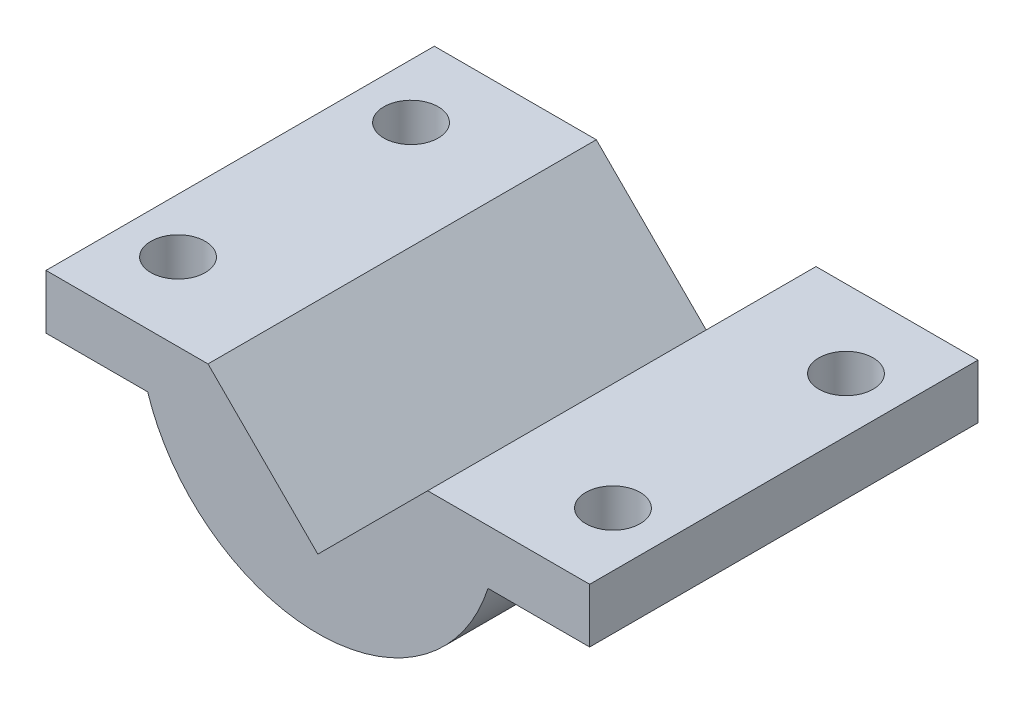
SolidWorks part; units mm, degrees
material "Plain Carbon Steel"
ref_plane "Front Plane" through (0, 0, 0) normal (0, 0, 1) x (1, 0, 0)
ref_plane "Top Plane" through (0, 0, 0) normal (0, 1, 0) x (1, 0, 0)
ref_plane "Right Plane" through (0, 0, 0) normal (1, 0, 0) x (0, 0, -1)
sketch "Saddle Profile Sketch" plane through (0, 0, 0) normal (0, 0, 1) x (1, 0, 0)
  line L0 (0, 25.7801) -> (0, -31.0664) construction
  line L1 (-51.6368, 0) -> (50.3344, 0) construction
  line L2 (0, 14.1421) -> (-14.1421, 0) construction
  line L3 (0, 14.1421) -> (14.1421, 0) construction
  line L4 (0, -14.1421) -> (14.1421, 0)
  line L5 (0, -14.1421) -> (-14.1421, 0)
  line L6 (-14.1421, 0) -> (-35, 0)
  line L7 (-35, 0) -> (-35, -7)
  line L8 (-35, -7) -> (-21.9089, -7)
  line L9 (35, -7) -> (21.9089, -7)
  line L10 (35, 0) -> (35, -7)
  line L11 (14.1421, 0) -> (35, 0)
  arc A0 (-21.9089, -7) -> (21.9089, -7) centre (0, 0) ccw
  dimension "D3" = 46
  dimension "D1" = 20
  dimension "D2" = 45
  dimension "D4" = 7
  dimension "D5" = 70
extrude "Saddle Body" add sketch "Saddle Profile Sketch" along normal mid plane 50
sketch "Flange Holes Sketch" plane through (0, 0, 0) normal (0, 1, 0) x (1, 0, 0)
  line L0 (0, 25) -> (0, 0) construction
  line L1 (0, -25) -> (0, 25) construction
  line L2 (0, 0) -> (-27.9707, 0) construction
  line L4 (-35, -25) -> (-35, 25) construction
  circle A0 centre (-28, 15) radius 3.5
  circle A1 centre (-28, -15) radius 3.5
  circle A2 centre (28, -15) radius 3.5
  circle A3 centre (28, 15) radius 3.5
  dimension "D2" = 7
  dimension "D1" = 7
  dimension "D4" = 15
  dimension "D5" = 15
  dimension "D3" = 2
extrude "Flange Mounting Holes" cut sketch "Flange Holes Sketch" against normal up to next
